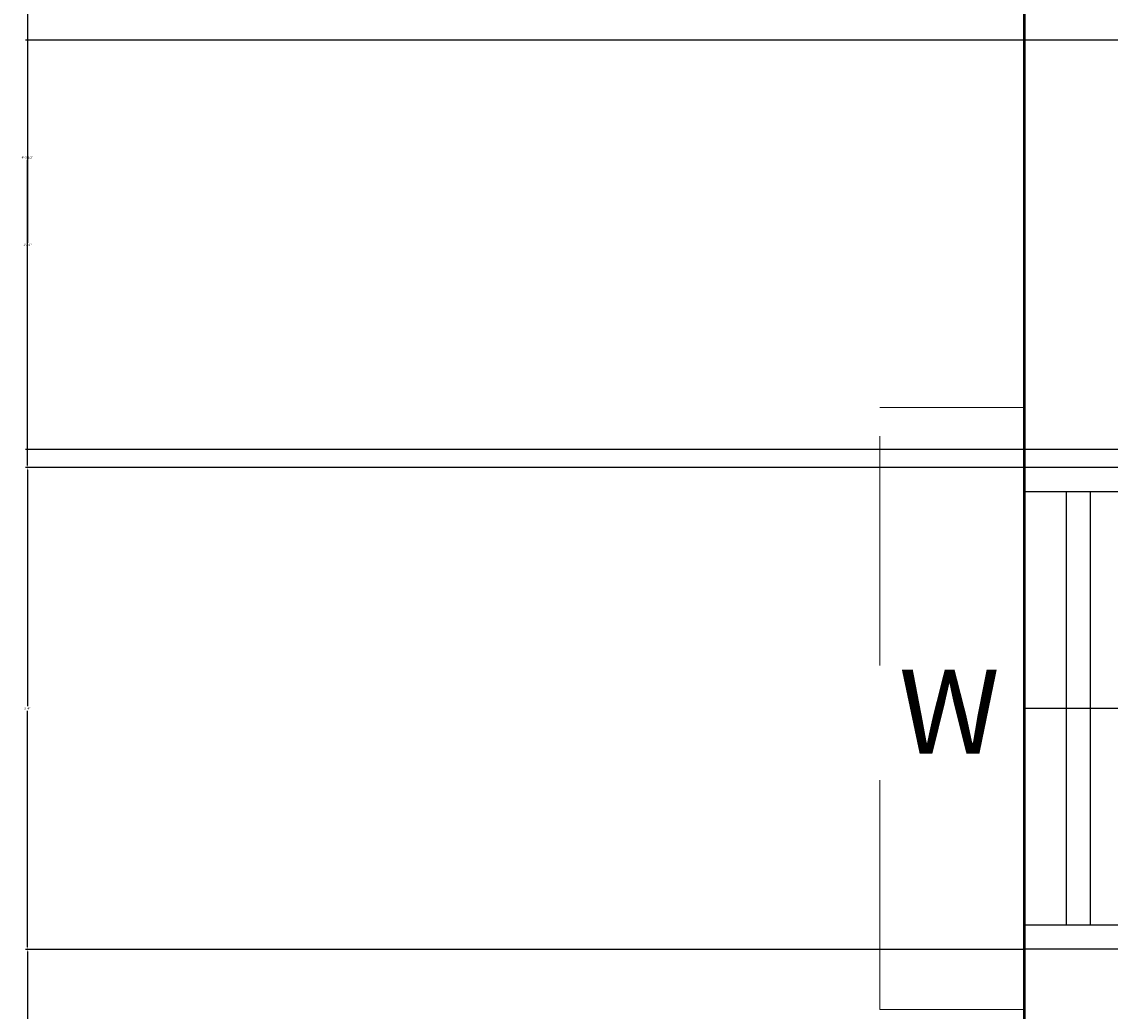
# Model space of a CAD drawing. Units: inches. Extents: x 37 to 824, y -700 to 234.
# Tile 41 of 77: x 78 to 168, y -75 to 8. Entities that reach past the tile are written whole.
import ezdxf

# ---------------------------------------------------------------- set-up
doc = ezdxf.new("R2010")
doc.units = ezdxf.units.IN
doc.header["$MEASUREMENT"] = 0
doc.linetypes.add('DASHED', pattern=[19.05, 12.7, -6.35])
for name, color, linetype, lineweight in [('A-ANNO-DIMS', 2, 'Continuous', 18), ('A-ANNO-TEXT', 7, 'Continuous', 18), ('A-GLAZ', 4, 'Continuous', 25), ('A-ROOF-OVHD', 1, 'DASHED', 18), ('A-WALL', 2, 'Continuous', 50)]:
    doc.layers.add(name, color=color, linetype=linetype, lineweight=lineweight)
doc.styles.get("Standard").update_dxf_attribs({"font": 'arial.ttf'})
doc.dimstyles.get("Standard").update_dxf_attribs({"dimtxt": 0.18, "dimasz": 0.18, "dimexe": 0.18, "dimexo": 0.0625, "dimgap": 0.09, "dimtad": 0, "dimtih": 1, "dimtoh": 1, "dimdec": 1, "dimzin": 0, "dimdsep": 46, "dimlunit": 4, "dimtxsty": 'Standard', "dimcen": 0.09, "dimadec": 0, "dimazin": 0, "dimtfac": 1, "dimtdec": 1, "dimtofl": 0, "dimtmove": 0, "dimatfit": 3, "dimfxl": 1, "dimtolj": 1, "dimtzin": 0, "dimarcsym": 0})

# ---------------------------------------------------------------- blocks, each defined once
blk = doc.blocks.new('WIN-900')
for p, q in [((0, 9), (0, 0)), ((2, 9), (2, 0)), ((20, 9), (20, 0)), ((38, 9), (38, 0)), ((40, 9), (40, 0)), ((38, 5.5), (2, 5.5)), ((38, 3.5), (2, 3.5))]:
    blk.add_line(p, q)
blk = doc.blocks.new('*D53')
at = {"layer": 'A-ANNO-DIMS', "color": 0, "lineweight": -2, "ltscale": 0.5, "transparency": 16777216}
for p, q in [((161.015, 22.09), (78.159, 22.09)), ((78.339, 21.91), (78.339, -3.476)), ((78.339, -29.23), (78.339, -3.843)), ((161.015, -29.41), (78.159, -29.41))]:
    blk.add_line(p, q, dxfattribs=at)
at = {"layer": 'A-ANNO-DIMS', "color": 0, "ltscale": 0.5, "transparency": 16777216}
for points in [[(78.309, 21.91), (78.369, 21.91), (78.339, 22.09)], [(78.309, -29.23), (78.369, -29.23), (78.339, -29.41)]]:
    blk.add_solid(points, dxfattribs=at)
at = {"layer": 'Defpoints', "color": 0, "ltscale": 0.5, "transparency": 16777216}
for p in [(161.077, 22.09), (78.339, -29.41), (161.077, -29.41)]:
    blk.add_point(p, dxfattribs=at)
at = {"layer": 'A-ANNO-DIMS', "color": 0, "ltscale": 0.5, "transparency": 16777216, "insert": (78.339, -3.66), "char_height": 0.18, "attachment_point": 5}
blk.add_mtext('\\A1;4\'-3 1/2"', dxfattribs=at)
blk = doc.blocks.new('*D54')
at = {"layer": 'A-ANNO-DIMS', "color": 0, "lineweight": -2, "ltscale": 0.5, "transparency": 16777216}
for p, q in [((161.015, -29.41), (78.159, -29.41)), ((78.339, -29.59), (78.339, -49.228)), ((78.339, -69.23), (78.339, -49.592)), ((161.015, -69.41), (78.159, -69.41))]:
    blk.add_line(p, q, dxfattribs=at)
at = {"layer": 'A-ANNO-DIMS', "color": 0, "ltscale": 0.5, "transparency": 16777216}
for points in [[(78.309, -29.59), (78.369, -29.59), (78.339, -29.41)], [(78.309, -69.23), (78.369, -69.23), (78.339, -69.41)]]:
    blk.add_solid(points, dxfattribs=at)
at = {"layer": 'Defpoints', "color": 0, "ltscale": 0.5, "transparency": 16777216}
for p in [(161.077, -29.41), (78.339, -69.41), (161.077, -69.41)]:
    blk.add_point(p, dxfattribs=at)
at = {"layer": 'A-ANNO-DIMS', "color": 0, "ltscale": 0.5, "transparency": 16777216, "insert": (78.339, -49.41), "char_height": 0.18, "attachment_point": 5}
blk.add_mtext('\\A1;3\'-4"', dxfattribs=at)
blk = doc.blocks.new('*D55')
at = {"layer": 'A-ANNO-DIMS', "color": 0, "lineweight": -2, "ltscale": 0.5, "transparency": 16777216}
for p, q in [((161.015, -69.41), (78.159, -69.41)), ((78.339, -69.59), (78.339, -85.228)), ((78.339, -101.23), (78.339, -85.591)), ((161.015, -101.41), (78.159, -101.41))]:
    blk.add_line(p, q, dxfattribs=at)
at = {"layer": 'A-ANNO-DIMS', "color": 0, "ltscale": 0.5, "transparency": 16777216}
for points in [[(78.309, -69.59), (78.369, -69.59), (78.339, -69.41)], [(78.309, -101.23), (78.369, -101.23), (78.339, -101.41)]]:
    blk.add_solid(points, dxfattribs=at)
at = {"layer": 'Defpoints', "color": 0, "ltscale": 0.5, "transparency": 16777216}
for p in [(161.077, -69.41), (78.339, -101.41), (161.077, -101.41)]:
    blk.add_point(p, dxfattribs=at)
at = {"layer": 'A-ANNO-DIMS', "color": 0, "ltscale": 0.5, "transparency": 16777216, "insert": (78.339, -85.41), "char_height": 0.18, "attachment_point": 5}
blk.add_mtext('\\A1;2\'-8"', dxfattribs=at)
blk = doc.blocks.new('*D62')
at = {"layer": 'A-ANNO-DIMS', "color": 0, "lineweight": -2, "ltscale": 0.5, "transparency": 16777216}
for p, q in [((419.015, 6.09), (78.159, 6.09)), ((78.339, 5.91), (78.339, -10.728)), ((78.339, -27.73), (78.339, -11.091)), ((419.015, -27.91), (78.159, -27.91))]:
    blk.add_line(p, q, dxfattribs=at)
at = {"layer": 'A-ANNO-DIMS', "color": 0, "ltscale": 0.5, "transparency": 16777216}
for points in [[(78.309, 5.91), (78.369, 5.91), (78.339, 6.09)], [(78.309, -27.73), (78.369, -27.73), (78.339, -27.91)]]:
    blk.add_solid(points, dxfattribs=at)
at = {"layer": 'Defpoints', "color": 0, "ltscale": 0.5, "transparency": 16777216}
for p in [(419.077, 6.09), (78.339, -27.91), (419.077, -27.91)]:
    blk.add_point(p, dxfattribs=at)
at = {"layer": 'A-ANNO-DIMS', "color": 0, "ltscale": 0.5, "transparency": 16777216, "insert": (78.339, -10.91), "char_height": 0.18, "attachment_point": 5}
blk.add_mtext('\\A1;2\'-10"', dxfattribs=at)

msp = doc.modelspace()

# ---------------------------------------------------------------- linework, layer by layer
at = {"layer": 'A-ROOF-OVHD', "ltscale": 1.5}
for p, q in [((161.077, -24.41), (149.077, -24.41)), ((149.077, -74.41), (149.077, -24.41)), ((161.077, -29.41), (161.077, -24.41)), ((161.077, -69.41), (161.077, -74.41)), ((161.077, -74.41), (149.077, -74.41))]:
    msp.add_line(p, q, dxfattribs=at)
at = {"layer": 'A-WALL'}
msp.add_line((161.077, 75.09), (161.077, -365.91), dxfattribs=at)

# ---------------------------------------------------------------- block references
at = {"layer": 'A-GLAZ', "rotation": 269.9999999999999}
msp.add_blockref('WIN-900', (161.077, -29.409), dxfattribs=at)

# ---------------------------------------------------------------- texts
at = {"layer": 'A-ANNO-TEXT'}
msp.add_text('W', height=7, dxfattribs=at).set_placement((150.667, -53.175))

# ---------------------------------------------------------------- dimensions: what is measured, and where the dimension line sits
at = {"layer": 'A-ANNO-DIMS', "ltscale": 0.5}
for base, p1, p2, picture, middle in [((78.339, -29.41), (161.077, 22.09), (161.077, -29.41), '*D53', (78.339, -3.66)), ((78.339, -27.91), (419.077, 6.09), (419.077, -27.91), '*D62', (78.339, -10.91)), ((78.339, -69.41), (161.077, -29.41), (161.077, -69.41), '*D54', (78.339, -49.41)), ((78.339, -101.41), (161.077, -69.41), (161.077, -101.41), '*D55', (78.339, -85.41))]:
    dim = msp.add_linear_dim(base=base, p1=p1, p2=p2, angle=90, dimstyle='Standard', override={"dimdec": 1, "dimlfac": 1, "dimrnd": 0, "dimzin": 1, "dimdsep": 46, "dimlunit": 4, "dimfrac": 2}, dxfattribs=at)
    dim.commit()
    dim.dimension.update_dxf_attribs({"geometry": picture, "text_midpoint": middle})

doc.saveas('drawing.dxf')
